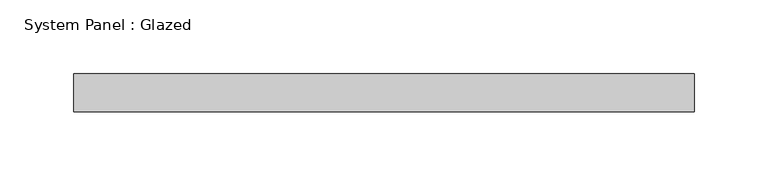
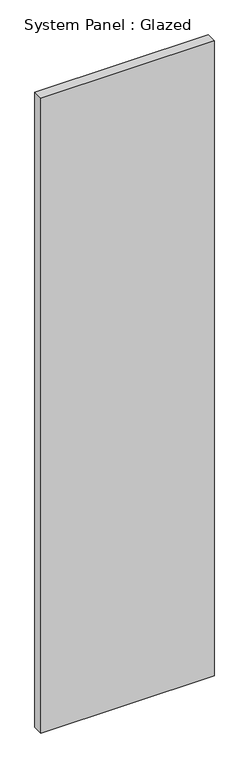
"""IFC4 building model written with IfcOpenShell, lengths in millimetres: plate geometry, System Panel : Glazed."""

from ifc_helpers import new_model, si_unit, origin, origin_with_axes, place, context, project, spatial, polyline, outline, extrude, source, transform, mapped, element, save


def system_panel_glazed_8b35a0ff(model_context):
    return source(origin(), model_context, "Body", "SweptSolid", [
        extrude(outline(polyline([(209.6599961, 19.05), (-209.6599961, 19.05), (-209.6599961, 44.45), (209.6599961, 44.45), (209.6599961, 19.05)])), origin_with_axes(), (0.0, 0.0, 1.0), 1625.6),
    ])


if __name__ == "__main__":
    model = new_model("IFC4")
    model_context = context("Model", 3, world=origin())
    ifc_project = project(units=[si_unit("LENGTHUNIT", "METRE", prefix="MILLI")], contexts=[model_context])
    site = spatial("IfcSite", under=ifc_project)
    building = spatial("IfcBuilding", under=site)
    placement = place(None, origin())
    system_panel_glazed_shape = system_panel_glazed_8b35a0ff(model_context)
    element("IfcPlate", 1, ObjectType="System Panel : Glazed", at=placement, inside=building, context=model_context, shape_type="MappedRepresentation", body=[
        mapped(system_panel_glazed_shape, transform((0.0, 0.0, 0.0), x_axis=(1.0, 0.0, 0.0), y_axis=(0.0, 1.0, 0.0), z_axis=(0.0, 0.0, 1.0))),
    ])
    save(model, "model.ifc")

# Revit data of these elements
# Type "System Panel : Glazed"
#   Construction Type Id = "GSP4R"
#   Analytic Construction = "1/8 in Pilkington single glazing"
#   Visual Light Transmittance = 0.9
#   Solar Heat Gain Coefficient = 0.86
#   Heat Transfer Coefficient (U) = 1.18115 BTU/(h·ft²·°F)
# Element 1 (IfcPlate, "System Panel : Glazed")
#   Materials on its faces: "Glass"
# Materials
#   "Glass": class "Glass", colour RGB 0 128 192, transparency 0.75, Description = "Soda Lime Glass", Cost = 0
